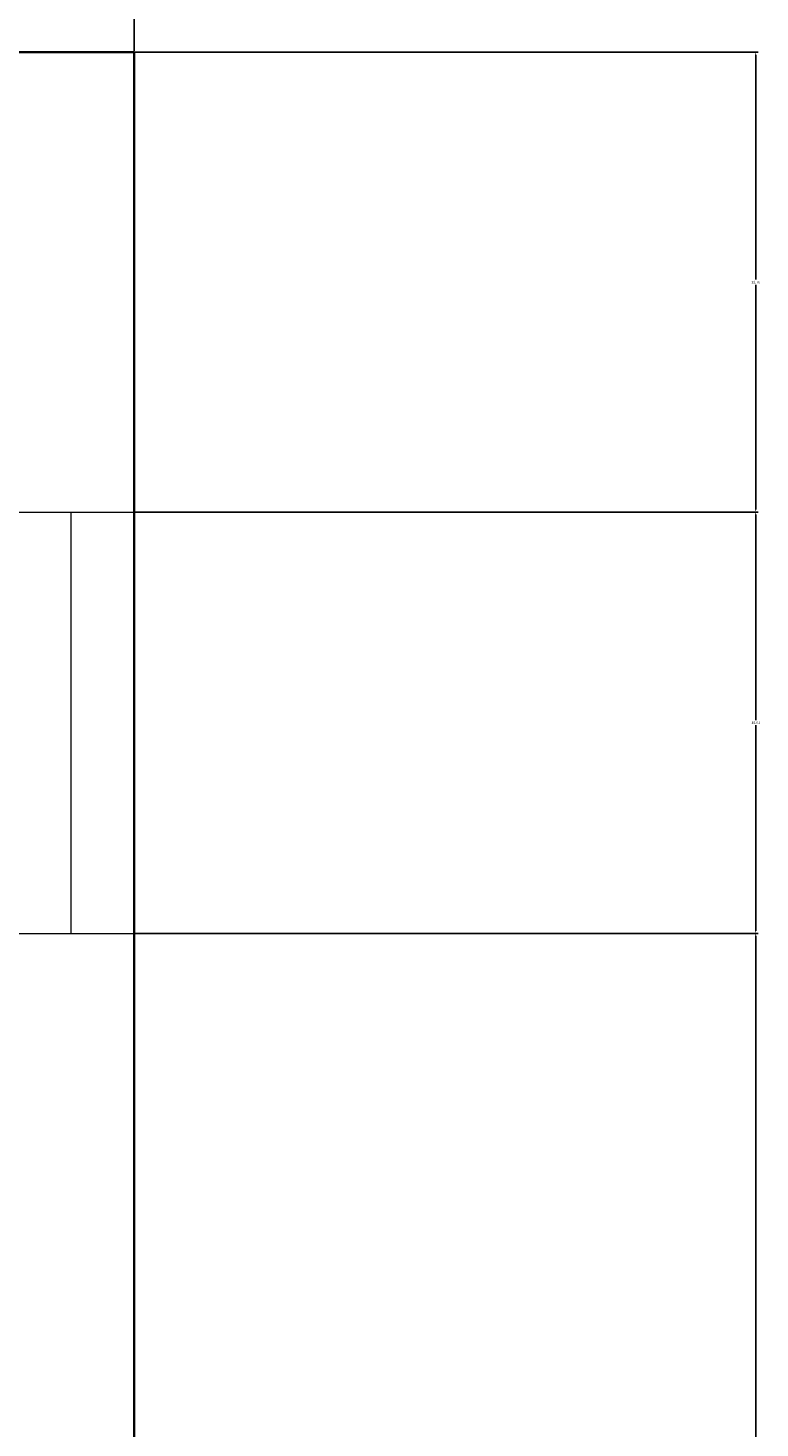
# Model space of a CAD drawing. Units: feet. Extents: x 2100 to 2836, y 2433 to 3396.
# Tile 10 of 12: x 2402 to 2454, y 3224 to 3324. Entities that reach past the tile are written whole.
import ezdxf

# ---------------------------------------------------------------- set-up
doc = ezdxf.new("R2010")
doc.units = ezdxf.units.FT
for name, color, linetype, lineweight in [('A-ANNO-DIMS', 2, 'Continuous', 18), ('A-GLAZ', 4, 'Continuous', 18), ('A-WALL', 7, 'Continuous', 35)]:
    doc.layers.add(name, color=color, linetype=linetype, lineweight=lineweight)
doc.styles.get("Standard").update_dxf_attribs({"font": 'arial.ttf'})
doc.dimstyles.get("Standard").update_dxf_attribs({"dimtxt": 0.18, "dimasz": 0.18, "dimexe": 0.18, "dimexo": 0.0625, "dimgap": 0.09, "dimtad": 0, "dimtih": 1, "dimtoh": 1, "dimdec": 4, "dimzin": 0, "dimdsep": 46, "dimtxsty": 'Standard', "dimcen": 0.09, "dimadec": 0, "dimazin": 0, "dimtfac": 1, "dimtdec": 4, "dimtofl": 0, "dimtmove": 0, "dimatfit": 3, "dimfxl": 1, "dimtolj": 1, "dimtzin": 0, "dimarcsym": 0})

# ---------------------------------------------------------------- blocks, each defined once
blk = doc.blocks.new('*D40')
at = {"layer": 'A-ANNO-DIMS', "color": 0, "lineweight": -2, "transparency": 16777216}
for p, q in [((2190.686, 3321.866), (2190.686, 3396.054)), ((2190.866, 3395.874), (2299.895, 3395.874)), ((2409.506, 3395.874), (2300.476, 3395.874)), ((2409.686, 3321.866), (2409.686, 3396.054))]:
    blk.add_line(p, q, dxfattribs=at)
at = {"layer": 'A-ANNO-DIMS', "color": 0, "transparency": 16777216}
for points in [[(2190.866, 3395.904), (2190.866, 3395.844), (2190.686, 3395.874)], [(2409.506, 3395.904), (2409.506, 3395.844), (2409.686, 3395.874)]]:
    blk.add_solid(points, dxfattribs=at)
at = {"layer": 'Defpoints', "color": 0, "transparency": 16777216}
for p in [(2409.686, 3395.874), (2190.686, 3321.803), (2409.686, 3321.803)]:
    blk.add_point(p, dxfattribs=at)
at = {"layer": 'A-ANNO-DIMS', "color": 0, "transparency": 16777216, "insert": (2300.186, 3395.874), "char_height": 0.18, "attachment_point": 5}
blk.add_mtext('\\A1;219', dxfattribs=at)
blk = doc.blocks.new('*D46')
at = {"layer": 'A-ANNO-DIMS', "color": 0, "lineweight": -2, "transparency": 16777216}
for p, q in [((2409.748, 3321.803), (2454.116, 3321.803)), ((2453.936, 3321.623), (2453.936, 3305.606)), ((2453.936, 3289.225), (2453.936, 3305.242)), ((2409.748, 3289.045), (2454.116, 3289.045))]:
    blk.add_line(p, q, dxfattribs=at)
at = {"layer": 'A-ANNO-DIMS', "color": 0, "transparency": 16777216}
for points in [[(2453.906, 3321.623), (2453.966, 3321.623), (2453.936, 3321.803)], [(2453.906, 3289.225), (2453.966, 3289.225), (2453.936, 3289.045)]]:
    blk.add_solid(points, dxfattribs=at)
at = {"layer": 'Defpoints', "color": 0, "transparency": 16777216}
for p in [(2409.686, 3321.803), (2409.686, 3289.045), (2453.936, 3289.045)]:
    blk.add_point(p, dxfattribs=at)
at = {"layer": 'A-ANNO-DIMS', "color": 0, "transparency": 16777216, "insert": (2453.936, 3305.424), "char_height": 0.18, "attachment_point": 5}
blk.add_mtext('\\A1;32.76', dxfattribs=at)
blk = doc.blocks.new('*D47')
at = {"layer": 'A-ANNO-DIMS', "color": 0, "lineweight": -2, "transparency": 16777216}
for p, q in [((2409.748, 3289.045), (2454.116, 3289.045)), ((2453.936, 3288.865), (2453.936, 3274.223)), ((2453.936, 3259.217), (2453.936, 3273.859)), ((2409.748, 3259.037), (2454.116, 3259.037))]:
    blk.add_line(p, q, dxfattribs=at)
at = {"layer": 'A-ANNO-DIMS', "color": 0, "transparency": 16777216}
for points in [[(2453.906, 3288.865), (2453.966, 3288.865), (2453.936, 3289.045)], [(2453.906, 3259.217), (2453.966, 3259.217), (2453.936, 3259.037)]]:
    blk.add_solid(points, dxfattribs=at)
at = {"layer": 'Defpoints', "color": 0, "transparency": 16777216}
for p in [(2409.686, 3289.045), (2409.686, 3259.037), (2453.936, 3259.037)]:
    blk.add_point(p, dxfattribs=at)
at = {"layer": 'A-ANNO-DIMS', "color": 0, "transparency": 16777216, "insert": (2453.936, 3274.041), "char_height": 0.18, "attachment_point": 5}
blk.add_mtext('\\A1;30.01', dxfattribs=at)
blk = doc.blocks.new('*D48')
at = {"layer": 'A-ANNO-DIMS', "color": 0, "lineweight": -2, "transparency": 16777216}
for p, q in [((2409.748, 3259.037), (2454.116, 3259.037)), ((2453.936, 3258.857), (2453.936, 3196.118)), ((2453.936, 3133.015), (2453.936, 3195.754)), ((2409.748, 3132.835), (2454.116, 3132.835))]:
    blk.add_line(p, q, dxfattribs=at)
at = {"layer": 'A-ANNO-DIMS', "color": 0, "transparency": 16777216}
for points in [[(2453.906, 3258.857), (2453.966, 3258.857), (2453.936, 3259.037)], [(2453.906, 3133.015), (2453.966, 3133.015), (2453.936, 3132.835)]]:
    blk.add_solid(points, dxfattribs=at)
at = {"layer": 'Defpoints', "color": 0, "transparency": 16777216}
for p in [(2409.686, 3259.037), (2409.686, 3132.835), (2453.936, 3132.835)]:
    blk.add_point(p, dxfattribs=at)
at = {"layer": 'A-ANNO-DIMS', "color": 0, "transparency": 16777216, "insert": (2453.936, 3195.936), "char_height": 0.18, "attachment_point": 5}
blk.add_mtext('\\A1;126.2', dxfattribs=at)

msp = doc.modelspace()

# ---------------------------------------------------------------- linework, layer by layer
at = {"layer": 'A-GLAZ'}
for p, q in [((2400.6857, 3289.0453), (2409.6857, 3289.0453)), ((2405.1857, 3289.0453), (2405.1857, 3259.0368)), ((2400.6857, 3259.0368), (2409.6857, 3259.0368))]:
    msp.add_line(p, q, dxfattribs=at)
at = {"layer": 'A-WALL'}
for p, q in [((2190.6857, 3321.8031), (2409.6857, 3321.8031)), ((2409.6857, 3321.8031), (2409.6857, 3232.8031)), ((2409.6857, 3321.8031), (2409.6857, 3171.8031))]:
    msp.add_line(p, q, dxfattribs=at)

# ---------------------------------------------------------------- dimensions: what is measured, and where the dimension line sits
at = {"layer": 'A-ANNO-DIMS'}
dim = msp.add_linear_dim(base=(2409.6857, 3395.8745), p1=(2190.6857, 3321.8031), p2=(2409.6857, 3321.8031), dimstyle='Standard', override={"dimdec": 0, "dimlfac": 1, "dimrnd": 0, "dimzin": 0, "dimdsep": 46, "dimlunit": 2}, dxfattribs=at)
dim.commit()
dim.dimension.update_dxf_attribs({"geometry": '*D40', "text_midpoint": (2300.1857, 3395.8745)})
for base, p1, p2, override, picture, middle in [((2453.9357, 3289.0453), (2409.6857, 3321.8031), (2409.6857, 3289.0453), {"dimdec": 2, "dimlfac": 1, "dimrnd": 0, "dimzin": 0, "dimdsep": 46, "dimlunit": 2}, '*D46', (2453.9357, 3305.4242)), ((2453.9357, 3259.0368), (2409.6857, 3289.0453), (2409.6857, 3259.0368), {"dimdec": 2, "dimlfac": 1, "dimrnd": 0, "dimzin": 0, "dimdsep": 46, "dimlunit": 2}, '*D47', (2453.9357, 3274.041)), ((2453.9357, 3132.8348), (2409.6857, 3259.0368), (2409.6857, 3132.8348), {"dimdec": 1, "dimlfac": 1, "dimrnd": 0, "dimzin": 0, "dimdsep": 46, "dimlunit": 2}, '*D48', (2453.9357, 3195.9358))]:
    dim = msp.add_linear_dim(base=base, p1=p1, p2=p2, angle=90, dimstyle='Standard', override=override, dxfattribs=at)
    dim.commit()
    dim.dimension.update_dxf_attribs({"geometry": picture, "text_midpoint": middle})

doc.saveas('drawing.dxf')
